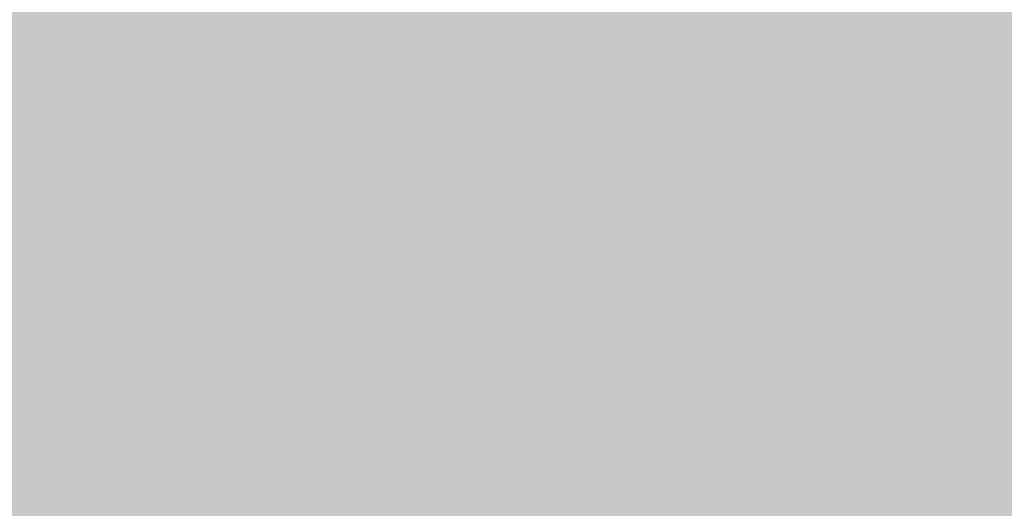
# Model space of a CAD drawing. Units: inches. Extents: x 2083 to 3317, y 1141 to 2115.
# Tile 159 of 256: x 3126.955939 to 3126.958245, y 1263.262504 to 1263.263648. Entities that reach past the tile are written whole.
import ezdxf

# ---------------------------------------------------------------- set-up
doc = ezdxf.new("R2010")
doc.units = ezdxf.units.IN
doc.layers.add('A-WALL-PATT', color=251, linetype='Continuous', lineweight=13, true_color=0x636466)

msp = doc.modelspace()

# ---------------------------------------------------------------- hatches: boundary and pattern name
at = {"layer": 'A-WALL-PATT'}
h = msp.add_hatch(color=256, dxfattribs=at)
h.dxf.hatch_style = 1
h.paths.add_polyline_path([(3126.9597832, 2020.7613601), (2748.9597832, 2020.7613601), (2604.9597832, 2020.7613601), (2226.9597832, 2020.7613601), (2226.9597832, 1702.7613601), (2466.9597832, 1702.7613601), (2466.9597832, 1582.7613601), (2418.9597832, 1582.7613601), (2418.9597832, 1477.7613601), (2226.9597832, 1477.7613601), (2226.9597832, 1263.2613601), (2544.9597832, 1263.2613601), (2544.9597832, 1411.7613601), (2604.9597832, 1411.7613601), (2685.9597832, 1411.7613601), (2685.9597832, 1420.7613601), (2604.9597832, 1420.7613601), (2604.9597832, 1573.7613601), (2604.9597832, 1702.7613601), (2604.9597832, 2011.7613601), (2748.9597832, 2011.7613601), (2748.9597832, 1702.7613601), (2862.9597832, 1702.7613601), (2862.9597832, 1621.7613601), (2871.9597832, 1621.7613601), (2871.9597832, 1702.7613601), (2883.9597832, 1702.7613601), (2883.9597832, 1706.9394595, -0.026459), (2883.9597832, 1711.7613601), (2757.9597832, 1711.7613601), (2757.9597832, 1807.7613601), (2787.9597832, 1807.7613601), (2787.9597832, 1812.2613601), (2757.9597832, 1812.2613601), (2757.9597832, 2011.7613601), (2877.9597832, 2011.7613601), (2877.9597832, 1812.2613601), (2847.9597832, 1812.2613601), (2847.9597832, 1807.7613601), (2889.8357425, 1807.7613601), (2889.8357425, 1812.2613601), (2882.4597832, 1812.2613601), (2882.4597832, 2011.7613601), (3117.9597832, 2011.7613601), (3117.9597832, 1812.2613601), (2937.8357425, 1812.2613601), (2937.8357425, 1807.7613601), (2995.7097832, 1807.7613601), (2995.7097832, 1796.1176655), (3000.2097832, 1796.1176655), (3000.2097832, 1807.7613601), (3117.9597832, 1807.7613601), (3117.9597832, 1711.7613601), (3000.2097832, 1711.7613601), (3000.2097832, 1760.1176655), (2998.5727047, 1760.1176655, -0.020711), (2995.7097832, 1760.1176655), (2995.7097832, 1711.7613601), (2931.9597832, 1711.7613601), (2931.9597832, 1702.7613601), (3126.9597832, 1702.7613601)])
h.paths.add_polyline_path([(2471.4597832, 2011.7613601), (2471.4597832, 1810.0113601), (2462.7169357, 1810.0113601), (2462.7169357, 1805.5113601), (2505.9597832, 1805.5113601), (2505.9597832, 1810.0113601), (2475.9597832, 1810.0113601), (2475.9597832, 2011.7613601), (2595.9597832, 2011.7613601), (2595.9597832, 1810.0113601), (2565.9597832, 1810.0113601), (2565.9597832, 1805.5113601), (2595.9597832, 1805.5113601), (2595.9597832, 1711.7613601), (2235.9597832, 1711.7613601), (2235.9597832, 1805.5113601), (2353.7097832, 1805.5113601), (2353.7097832, 1796.0541624), (2358.2097832, 1796.0541624), (2358.2097832, 1805.5113601), (2414.7169357, 1805.5113601), (2414.7169357, 1810.0113601), (2235.9597832, 1810.0113601), (2235.9597832, 2011.7613601)], flags=16)
h.paths.add_polyline_path([(2270.2047343, 1994.6100082), (2270.2047343, 1970.6100082), (2246.2047343, 1970.6100082), (2246.2047343, 1994.6100082)], flags=0)
edge = h.paths.add_edge_path(flags=0)
edge.add_ellipse((2332.027391, 1899.7981761), major_axis=(-3.0429938, 3.0429938), ratio=0.16825245, start_angle=-161.3321656, end_angle=-156.3071136, ccw=False)
edge.add_ellipse((2333.0820373, 1898.7435297), major_axis=(-1.0546463, 1.0546463), ratio=0.453532097, start_angle=-123.371019, end_angle=-94.1591066)
edge = h.paths.add_edge_path(flags=0)
edge.add_ellipse((2332.027391, 1968.8762897), major_axis=(3.0429938, 3.0429938), ratio=0.16825245, start_angle=18.6678344, end_angle=23.6928864)
edge.add_spline(control_points=[(2332.9255964, 1970.6911045), (2332.2267681, 1970.3360997), (2330.8937087, 1969.6589054), (2328.4130803, 1970.9321376), (2327.2039345, 1967.7487119), (2324.7095965, 1969.9555886), (2322.5328223, 1967.012354), (2320.0128462, 1971.2958124), (2317.6803077, 1968.1578449), (2316.0405263, 1967.1020468), (2315.4269045, 1966.8096022)], knot_values=[0, 0, 0, 0, 2.267059, 4.324559, 6.685584, 8.878641, 11.121502, 14.300359, 17.755284, 19.732645, 19.732645, 19.732645, 19.732645], degree=3, periodic=0)
edge.add_ellipse((2332.027391, 1968.8762897), major_axis=(3.0429938, 3.0429938), ratio=0.16825245, start_angle=18.6678344, end_angle=23.6928864, ccw=False)
edge.add_ellipse((2333.0820373, 1969.930936), major_axis=(1.0546463, 1.0546463), ratio=0.453532097, start_angle=56.628981, end_angle=85.8408934, ccw=False)
edge = h.paths.add_edge_path(flags=0)
edge.add_spline(control_points=[(2296.4282874, 1967.9879081), (2293.6278045, 1965.3363137), (2287.7036238, 1959.727094), (2299.7438601, 1949.9956993), (2294.5325909, 1935.6685275), (2290.5732281, 1920.6035119), (2293.3941244, 1909.9736911), (2296.1854073, 1904.9665431)], knot_values=[0.099185, 0.099185, 0.099185, 0.099185, 0.345301, 0.619822, 0.982653, 1.386093, 1.810555, 1.810555, 1.810555, 1.810555], degree=3, periodic=0)
edge.add_spline(control_points=[(2296.1854073, 1904.9665431), (2297.3835817, 1902.6193002), (2298.0009694, 1901.9493116), (2298.5529698, 1901.4681549)], knot_values=[0.006246, 0.006246, 0.006246, 0.006246, 0.055476, 0.055476, 0.055476, 0.055476], degree=3, periodic=0)
edge.add_spline(control_points=[(2298.5529698, 1901.4681549), (2297.2586121, 1900.9232238), (2295.2252939, 1900.2321257), (2293.0602287, 1900.6142053), (2292.1014227, 1900.788415), (2292.0895776, 1900.790568)], knot_values=[0.312835, 0.312835, 0.312835, 0.312835, 0.40178, 0.474987, 0.475903, 0.475903, 0.475903, 0.475903], degree=3, periodic=0)
edge.add_arc((2292.7936464, 1904.6641088), 3.9370079, 215.4208969, 259.6981795, ccw=False)
edge.add_spline(control_points=[(2289.5853139, 1902.3823039), (2289.4766524, 1902.5350874), (2289.3684805, 1902.6880353), (2289.2608648, 1902.8411699)], knot_values=[0.102872, 0.102872, 0.102872, 0.102872, 0.116896, 0.116896, 0.116896, 0.116896], degree=3, periodic=0)
edge.add_spline(control_points=[(2289.2608648, 1902.8411699), (2288.6866042, 1902.5501922), (2287.6400477, 1902.0199025), (2285.8813368, 1901.8739536), (2283.8529717, 1901.5043521), (2281.7199871, 1899.7105375), (2278.4669913, 1899.492942), (2276.1571361, 1901.8832022), (2272.2589526, 1899.8040711), (2267.7776054, 1901.8431828), (2262.2438819, 1900.1840326), (2257.414927, 1901.7820606), (2254.318374, 1900.7261196), (2253.1782849, 1900.3373431)], knot_values=[0, 0, 0, 0, 1.907977, 3.477176, 5.261074, 7.972851, 11.680248, 13.717921, 16.939592, 22.789562, 27.502503, 33.595215, 37.145618, 37.145618, 37.145618, 37.145618], degree=3, periodic=0)
edge.add_line((2253.1782849, 1900.3373431), (2250.2442397, 1902.8411699))
edge.add_line((2250.2442397, 1902.8411699), (2250.2442397, 1965.8332959))
edge.add_line((2250.2442397, 1965.8332959), (2253.1782849, 1968.3371226))
edge.add_spline(control_points=[(2253.1782849, 1968.3371226), (2254.318374, 1967.9483462), (2257.414927, 1966.8924051), (2262.2438819, 1968.4904332), (2267.7776054, 1966.8312829), (2271.5267301, 1968.5372172), (2273.8759143, 1967.8282895), (2274.2067012, 1967.7276424)], knot_values=[0, 0, 0, 0, 0.09018, 0.244935, 0.364644, 0.513233, 0.537855, 0.537855, 0.537855, 0.537855], degree=3, periodic=0)
edge.add_arc((2274.3528869, 1963.7933495), 3.9370079, 72.0511336, 92.1279492, ccw=False)
edge.add_arc((2281.2969331, 1985.2300027), 18.5962982, 252.05113361, 288.56572166)
edge.add_arc((2292.3167172, 1956.0288805), 12.6460805, 71.02678788, 113.77821843, ccw=False)
edge = h.paths.add_edge_path(flags=0)
edge.add_spline(control_points=[(2274.8994147, 1951.8561946), (2275.066156, 1951.6165924), (2275.2326866, 1951.3765878), (2275.3979871, 1951.1358545)], knot_values=[1.409916, 1.409916, 1.409916, 1.409916, 1.43159, 1.43159, 1.43159, 1.43159], degree=3, periodic=0)
edge.add_spline(control_points=[(2275.3979871, 1951.1358545), (2275.7921055, 1950.5618854), (2276.1792311, 1949.9837745), (2276.5455462, 1949.3971029)], knot_values=[1.358238, 1.358238, 1.358238, 1.358238, 1.409916, 1.409916, 1.409916, 1.409916], degree=3, periodic=0)
edge.add_line((2276.5455462, 1949.3971029), (2277.437289, 1947.8621847))
edge.add_spline(control_points=[(2277.437289, 1947.8621847), (2276.3038341, 1945.6731147), (2274.6396979, 1942.4268817), (2274.631615, 1938.0938998), (2272.7991237, 1930.8515498), (2274.3564261, 1943.8970461), (2275.9476814, 1947.9233558), (2276.5455462, 1949.3971029)], knot_values=[0.005632, 0.005632, 0.005632, 0.005632, 0.186014, 0.266002, 0.357087, 0.59639, 0.739732, 0.739732, 0.739732, 0.739732], degree=3, periodic=0)
edge.add_spline(control_points=[(2276.5455462, 1949.3971029), (2276.1792311, 1949.9837745), (2275.7921055, 1950.5618854), (2275.3979871, 1951.1358545)], knot_values=[1.358238, 1.358238, 1.358238, 1.358238, 1.409916, 1.409916, 1.409916, 1.409916], degree=3, periodic=0)
edge.add_spline(control_points=[(2275.3979871, 1951.1358545), (2274.9425002, 1950.0804523), (2274.2077604, 1948.0252718), (2273.9346018, 1944.8514774), (2272.4685341, 1937.6274891), (2273.4662155, 1945.6964663), (2274.7006154, 1951.0594725), (2274.8994147, 1951.8561946)], knot_values=[0.104364, 0.104364, 0.104364, 0.104364, 0.189636, 0.269624, 0.36071, 0.600013, 0.644622, 0.644622, 0.644622, 0.644622], degree=3, periodic=0)
h.paths.add_polyline_path([(2269.1675139, 1963.1275729, -0.357527), (2268.170633, 1960.9763695, -0.092561), (2268.170633, 1939.4363249, -0.357527), (2269.1675139, 1937.2851215, -0.357527), (2267.0163105, 1938.2820024, -0.164785), (2254.6855813, 1938.2820024, -0.357527), (2252.5343779, 1937.2851215, -0.357527), (2253.5312587, 1939.4363249, -0.092561), (2253.5312587, 1960.9763695, -0.357527), (2252.5343779, 1963.1275729, -0.357527), (2254.6855813, 1962.130692, -0.164785), (2267.0163105, 1962.130692, -0.357527)], flags=0)
h.paths.add_polyline_path([(2248.8740679, 1967.8017998), (2248.8740679, 1957.0277095), (2249.4577833, 1957.0277095), (2249.4577833, 1911.6467562), (2248.8740679, 1911.6467562), (2248.8740679, 1900.8726659), (2246.5118632, 1900.8726659, 0.197327), (2244.1496584, 1902.4568734), (2244.1496584, 1966.2175923, 0.197327), (2246.5118632, 1967.8017998)], flags=0)
h.paths.add_polyline_path([(2269.1675139, 1931.3893442, -0.357527), (2268.170633, 1929.2381408, -0.092561), (2268.170633, 1907.6980962, -0.357527), (2269.1675139, 1905.5468928, -0.357527), (2267.0163105, 1906.5437737, -0.164785), (2254.6855813, 1906.5437737, -0.357527), (2252.5343779, 1905.5468928, -0.357527), (2253.5312587, 1907.6980962, -0.092561), (2253.5312587, 1929.2381408, -0.357527), (2252.5343779, 1931.3893442, -0.357527), (2254.6855813, 1930.3924634, -0.164785), (2267.0163105, 1930.3924634, -0.357527)], flags=0)
edge = h.paths.add_edge_path(flags=0)
edge.add_spline(control_points=[(2276.1968578, 1906.7237016), (2276.1681442, 1909.0289278), (2276.1140492, 1913.371852), (2270.5984171, 1924.9249783), (2273.9051746, 1919.0127787), (2275.9217115, 1916.2620626), (2275.4745699, 1912.4021495), (2277.2578735, 1910.3806206), (2276.6960436, 1908.2250358), (2276.6462176, 1906.8130226), (2276.6178249, 1906.0084068)], knot_values=[0, 0, 0, 0, 8.61026, 16.221274, 18.843057, 23.804898, 27.440828, 29.356102, 31.203478, 33.650687, 33.650687, 33.650687, 33.650687], degree=3, periodic=0)
edge.add_spline(control_points=[(2276.6178249, 1906.0084068), (2276.6233131, 1905.6241436), (2276.4977381, 1904.6286608), (2275.4417789, 1903.8547251), (2274.9373144, 1903.0804497), (2274.8590804, 1902.8411699)], knot_values=[0.156488, 0.156488, 0.156488, 0.156488, 0.184398, 0.231376, 0.250598, 0.250598, 0.250598, 0.250598], degree=3, periodic=0)
edge.add_line((2274.8590804, 1902.8411699), (2276.50598, 1902.8411699))
edge.add_spline(control_points=[(2276.50598, 1902.8411699), (2276.7883084, 1903.0849395), (2277.6650711, 1904.1251958), (2278.2495378, 1904.340738), (2277.6538719, 1908.5273866), (2278.15567, 1906.2278078), (2278.100464, 1905.2859484), (2278.8466748, 1904.0690054), (2277.8567853, 1903.4149482), (2277.8741909, 1902.9910497), (2277.9035616, 1902.8411699)], knot_values=[0.059574, 0.059574, 0.059574, 0.059574, 0.080753, 0.103741, 0.16972, 0.176036, 0.207137, 0.240474, 0.262341, 0.27366, 0.27366, 0.27366, 0.27366], degree=3, periodic=0)
edge.add_line((2277.9035616, 1902.8411699), (2280.0298255, 1902.8411699))
edge.add_spline(control_points=[(2280.0298255, 1902.8411699), (2279.8882214, 1903.088398), (2279.4992571, 1903.9815512), (2280.1522839, 1905.9393491), (2278.103615, 1909.6577572), (2279.7623946, 1907.185285), (2280.3279002, 1904.8748608), (2280.4851086, 1903.4895904), (2281.4632687, 1903.2494323), (2281.7583431, 1902.9364967), (2281.8340361, 1902.8411699)], knot_values=[0.013856, 0.013856, 0.013856, 0.013856, 0.034874, 0.088867, 0.107879, 0.126738, 0.158714, 0.193757, 0.217487, 0.226722, 0.226722, 0.226722, 0.226722], degree=3, periodic=0)
edge.add_spline(control_points=[(2281.8340361, 1902.8411699), (2281.7875348, 1902.8267029), (2281.6470224, 1902.7829881), (2281.3955272, 1902.85949), (2281.088077, 1902.9852418), (2280.7206826, 1903.060902), (2280.3334513, 1903.0257257), (2280.1247668, 1902.898879), (2280.0298255, 1902.8411699)], knot_values=[0, 0, 0, 0, 0.14413, 0.435517, 0.749276, 1.153046, 1.548371, 1.878348, 1.878348, 1.878348, 1.878348], degree=3, periodic=0)
edge.add_line((2280.0298255, 1902.8411699), (2277.9035616, 1902.8411699))
edge.add_spline(control_points=[(2277.9035616, 1902.8411699), (2277.892855, 1902.7958553), (2277.865396, 1902.6796374), (2277.6074793, 1902.6874828), (2277.2740503, 1902.8006999), (2276.8379209, 1902.6197745), (2276.5838074, 1902.7892611), (2276.50598, 1902.8411699)], knot_values=[0, 0, 0, 0, 0.127189, 0.326199, 0.628009, 1.24357, 1.515331, 1.515331, 1.515331, 1.515331], degree=3, periodic=0)
edge.add_line((2276.50598, 1902.8411699), (2274.8590804, 1902.8411699))
edge.add_spline(control_points=[(2274.8590804, 1902.8411699), (2274.8144367, 1902.8985868), (2274.7251297, 1903.013446), (2274.4934765, 1903.1189684), (2274.2442854, 1902.9605386), (2273.9371207, 1903.1849416), (2273.6140395, 1902.9831428), (2273.4083164, 1902.8830449), (2273.322254, 1902.8411699)], knot_values=[0, 0, 0, 0, 0.21843, 0.436957, 0.687977, 0.990379, 1.398396, 1.69185, 1.69185, 1.69185, 1.69185], degree=3, periodic=0)
edge.add_spline(control_points=[(2273.322254, 1902.8411699), (2273.6167403, 1903.445692), (2274.2739977, 1904.5382529), (2276.0272387, 1904.5737017), (2276.2069634, 1906.5836372), (2276.1968578, 1906.7237016)], knot_values=[0.012227, 0.012227, 0.012227, 0.012227, 0.059472, 0.106218, 0.134458, 0.134458, 0.134458, 0.134458], degree=3, periodic=0)
h.paths.add_polyline_path([(2270.7760538, 1897.7898284), (2270.7760538, 1873.7898284), (2246.7760538, 1873.7898284), (2246.7760538, 1897.7898284)], flags=0)
h.paths.add_polyline_path([(2353.7097832, 1760.0050593), (2353.7097832, 1760.0541624), (2358.2097832, 1760.0541624, -0.033729)], flags=0)
h.paths.add_polyline_path([(2321.8191188, 1737.5291862), (2341.9953271, 1737.5291862, -0.414214), (2343.2032727, 1736.3212406), (2343.2032727, 1721.0205964, -0.414214), (2341.9953271, 1719.8126508), (2321.8191188, 1719.8126508, -0.414214), (2320.6111732, 1721.0205964), (2320.6111732, 1736.3212406, -0.414214)], flags=0)
h.paths.add_polyline_path([(2324.2350099, 1736.3212406), (2339.5794359, 1736.3212406, -0.414214), (2341.9953271, 1733.9053494), (2341.9953271, 1725.4497302, -0.414214), (2339.5794359, 1723.033839), (2333.6805885, 1723.033839), (2333.8453172, 1722.0454666, -0.870646), (2335.4253988, 1721.8258934, -0.767327), (2333.922694, 1721.4232449), (2331.2910241, 1721.4232449, -0.767327), (2329.7883193, 1721.8258934, -0.870646), (2331.3684009, 1722.0454666), (2331.5331296, 1723.033839), (2324.2350099, 1723.033839, -0.414214), (2321.8191188, 1725.4497302), (2321.8191188, 1733.9053494, -0.414214)], flags=0)
h.paths.add_polyline_path([(2570.4837892, 1928.6154443), (2589.6837892, 1928.6154443), (2590.1688286, 1928.6154443), (2590.1688286, 1904.9933971), (2570.4837892, 1904.9933971)], flags=0)
h.paths.add_polyline_path([(2574.4473242, 1927.2638215, -1), (2572.8288357, 1927.2638215, -1)], flags=0)
h.paths.add_polyline_path([(2573.0898665, 1926.9408768), (2573.925032, 1927.7760423), (2574.1477428, 1927.5533315), (2573.3125773, 1926.718166)], flags=0)
h.paths.add_polyline_path([(2578.7790648, 1919.7296175, -1), (2571.5916632, 1919.7296175, -1)], flags=0)
h.paths.add_polyline_path([(2578.385364, 1919.7296175, -1), (2571.985364, 1919.7296175, -1)], flags=0)
h.paths.add_polyline_path([(2331.5957638, 1729.4762156, -1), (2333.6179542, 1729.4762156, -1)], flags=0)
h.paths.add_polyline_path([(2578.0342282, 1927.2638215, -1), (2576.4157396, 1927.2638215, -1)], flags=0)
h.paths.add_polyline_path([(2576.6888513, 1927.5310886), (2576.9115621, 1927.7537993), (2577.7467276, 1926.9186339), (2577.5240168, 1926.6959231)], flags=0)
h.paths.add_polyline_path([(2578.1390648, 1909.8595388, -1), (2572.2316632, 1909.8595388, -1)], flags=0)
h.paths.add_polyline_path([(2577.745364, 1909.8595388, -1), (2572.625364, 1909.8595388, -1)], flags=0)
h.paths.add_polyline_path([(2583.7977179, 1927.2638215, -1), (2582.1792294, 1927.2638215, -1)], flags=0)
h.paths.add_polyline_path([(2582.7186487, 1927.7537993), (2583.5538142, 1926.9186339), (2583.3311034, 1926.6959231), (2582.4959379, 1927.5310886)], flags=0)
h.paths.add_polyline_path([(2582.4959379, 1927.5310886), (2582.7186487, 1927.7537993), (2583.5538142, 1926.9186339), (2583.3311034, 1926.6959231)], flags=0)
h.paths.add_polyline_path([(2587.7390648, 1920.5296175, -1), (2581.8316632, 1920.5296175, -1)], flags=0)
h.paths.add_polyline_path([(2587.345364, 1920.5296175, -1), (2582.225364, 1920.5296175, -1)], flags=0)
h.paths.add_polyline_path([(2587.3846219, 1927.2638215, -1), (2585.7661333, 1927.2638215, -1)], flags=0)
h.paths.add_polyline_path([(2586.0819925, 1926.9802469), (2586.917158, 1927.8154124), (2587.1398688, 1927.5927016), (2586.3047033, 1926.7575361)], flags=0)
h.paths.add_polyline_path([(2588.3790648, 1910.6595388, -1), (2581.1916632, 1910.6595388, -1)], flags=0)
h.paths.add_polyline_path([(2587.985364, 1910.6595388, -1), (2581.585364, 1910.6595388, -1)], flags=0)
h.paths.add_polyline_path([(2417.1677288, 1729.4778955), (2437.3439372, 1729.4778955, -0.414214), (2438.5518828, 1728.2699499), (2438.5518828, 1712.9693057, -0.414214), (2437.3439372, 1711.7613601), (2417.1677288, 1711.7613601, -0.414214), (2415.9597832, 1712.9693057), (2415.9597832, 1728.2699499, -0.414214)], flags=0)
h.paths.add_polyline_path([(2419.58362, 1728.2699499), (2434.928046, 1728.2699499, -0.414214), (2437.3439372, 1725.8540587), (2437.3439372, 1717.3984395, -0.414214), (2434.928046, 1714.9825483), (2429.0291985, 1714.9825483), (2429.1939273, 1713.9941758, -0.870646), (2430.7740089, 1713.7746027, -0.767327), (2429.2713041, 1713.3719542), (2426.6396342, 1713.3719542, -0.767327), (2425.1369294, 1713.7746027, -0.870646), (2426.717011, 1713.9941758), (2426.8817397, 1714.9825483), (2419.58362, 1714.9825483, -0.414214), (2417.1677288, 1717.3984395), (2417.1677288, 1725.8540587, -0.414214)], flags=0)
h.paths.add_polyline_path([(2419.58362, 1728.2699499), (2434.928046, 1728.2699499, -0.414214), (2437.3439372, 1725.8540587), (2437.3439372, 1717.3984395, -0.414214), (2434.928046, 1714.9825483), (2429.0291985, 1714.9825483), (2428.3581177, 1719.0090337), (2427.5528206, 1719.0090337), (2426.8817397, 1714.9825483), (2419.58362, 1714.9825483, -0.414214), (2417.1677288, 1717.3984395), (2417.1677288, 1725.8540587, -0.414214)], flags=0)
h.paths.add_polyline_path([(2426.9443739, 1721.4249248, -1), (2428.9665643, 1721.4249248, -1)], flags=0)
h.paths.add_polyline_path([(2475.9597832, 1702.7613601), (2595.9597832, 1702.7613601), (2595.9597832, 1582.7613601), (2475.9597832, 1582.7613601)], flags=16)
h.paths.add_polyline_path([(2427.9597832, 1573.7613601), (2595.9597832, 1573.7613601), (2595.9597832, 1468.7613601), (2595.9597832, 1420.7613601), (2384.4597832, 1420.7613601), (2384.4597832, 1468.7613601), (2427.9597832, 1468.7613601)], flags=16)
h.paths.add_polyline_path([(2379.9597832, 1468.7613601), (2379.9597832, 1420.7613601), (2235.9597832, 1420.7613601), (2235.9597832, 1468.7613601)], flags=16)
h.paths.add_polyline_path([(2317.8159962, 1466.695767), (2337.9922045, 1466.695767, -0.414214), (2339.2001501, 1465.4878214), (2339.2001501, 1450.1871771, -0.414214), (2337.9922045, 1448.9792315), (2317.8159962, 1448.9792315, -0.414214), (2316.6080506, 1450.1871771), (2316.6080506, 1465.4878214, -0.414214)], flags=0)
h.paths.add_polyline_path([(2320.2318874, 1465.4878214), (2335.5763133, 1465.4878214, -0.414214), (2337.9922045, 1463.0719302), (2337.9922045, 1454.616311, -0.414214), (2335.5763133, 1452.2004198), (2329.6774659, 1452.2004198), (2329.8421946, 1451.2120473, -0.870646), (2331.4222762, 1450.9924742, -0.767327), (2329.9195714, 1450.5898257), (2327.2879015, 1450.5898257, -0.767327), (2325.7851967, 1450.9924742, -0.870646), (2327.3652783, 1451.2120473), (2327.530007, 1452.2004198), (2320.2318874, 1452.2004198, -0.414214), (2317.8159962, 1454.616311), (2317.8159962, 1463.0719302, -0.414214)], flags=0)
h.paths.add_polyline_path([(2320.2318874, 1465.4878214), (2335.5763133, 1465.4878214, -0.414214), (2337.9922045, 1463.0719302), (2337.9922045, 1454.616311, -0.414214), (2335.5763133, 1452.2004198), (2329.6774659, 1452.2004198), (2329.006385, 1456.2269051), (2328.2010879, 1456.2269051), (2327.530007, 1452.2004198), (2320.2318874, 1452.2004198, -0.414214), (2317.8159962, 1454.616311), (2317.8159962, 1463.0719302, -0.414214)], flags=0)
h.paths.add_polyline_path([(2327.5926413, 1458.6427963, -1), (2329.6148317, 1458.6427963, -1)], flags=0)
h.paths.add_polyline_path([(2244.4117436, 1433.3404531), (2241.9209449, 1433.3404531, -0.414214), (2240.0178562, 1435.2435418), (2240.0178562, 1440.9528078, -0.414211), (2241.920925, 1442.8558965), (2244.4117436, 1442.8558965, -1.976472)], flags=0)
h.paths.add_polyline_path([(2245.3568884, 1434.3975358, -0.414214), (2245.3568884, 1441.7988138, -2.144098)], flags=0)
h.paths.add_polyline_path([(2535.9597832, 1416.2613601), (2535.9597832, 1272.2613601), (2235.9597832, 1272.2613601), (2235.9597832, 1416.2613601)], flags=16)
h.paths.add_polyline_path([(2260.1195614, 1384.2928413), (2260.1195614, 1362.0386487), (2237.8653688, 1362.0386487), (2237.8653688, 1384.2928413)], flags=0)
edge = h.paths.add_edge_path(flags=0)
edge.add_line((2318.2518466, 1362.0932983), (2318.1457968, 1362.0009726))
edge.add_ellipse((2317.4451158, 1360.4310442), major_axis=(2.8216404, 2.8216404), ratio=0.16825245, start_angle=18.6678344, end_angle=20.9481273, ccw=False)
edge.add_ellipse((2318.4230451, 1361.4089735), major_axis=(0.9779293, 0.9779293), ratio=0.453532097, start_angle=56.628981, end_angle=70.2262012, ccw=False)
edge = h.paths.add_edge_path(flags=0)
edge.add_line((2319.1073699, 1295.5710784), (2319.0150442, 1295.6771282))
edge.add_ellipse((2317.4451158, 1296.3778091), major_axis=(-2.8216404, 2.8216404), ratio=0.16825245, start_angle=-161.3321656, end_angle=-159.0518727, ccw=False)
edge.add_ellipse((2318.4230451, 1295.3998798), major_axis=(-0.9779293, 0.9779293), ratio=0.453532097, start_angle=-123.371019, end_angle=-109.7737988)
edge = h.paths.add_edge_path(flags=0)
edge.add_spline(control_points=[(2284.2103489, 1301.1702189), (2284.5806878, 1300.444719), (2284.8911891, 1299.8920243), (2285.159553, 1299.4610182)], knot_values=[0.039066, 0.039066, 0.039066, 0.039066, 0.055476, 0.055476, 0.055476, 0.055476], degree=3, periodic=0)
edge.add_line((2285.159553, 1299.4610182), (2284.2103489, 1301.1702189))
edge = h.paths.add_edge_path(flags=0)
edge.add_line((2280.4124579, 1297.2980125), (2283.3699905, 1297.0361216))
edge.add_line((2283.3699905, 1297.0361216), (2286.4056902, 1297.9263104))
edge.add_spline(control_points=[(2286.4056902, 1297.9263104), (2285.305487, 1297.4631193), (2284.3447774, 1297.1291508), (2283.3699905, 1297.0361216)], knot_values=[0.394369, 0.394369, 0.394369, 0.394369, 0.475903, 0.475903, 0.475903, 0.475903], degree=3, periodic=0)
edge.add_spline(control_points=[(2283.3699905, 1297.0361216), (2283.2813895, 1297.027666), (2282.316289, 1296.9573356), (2281.3125019, 1297.1344787), (2280.4234414, 1297.2960161), (2280.4124579, 1297.2980125)], knot_values=[0.312835, 0.312835, 0.312835, 0.312835, 0.320246, 0.393453, 0.394369, 0.394369, 0.394369, 0.394369], degree=3, periodic=0)
edge = h.paths.add_edge_path(flags=0)
edge.add_line((2284.4355615, 1359.6072854), (2280.4462909, 1355.328047))
edge.add_line((2280.4462909, 1355.328047), (2279.5799868, 1351.0177544))
edge.add_line((2279.5799868, 1351.0177544), (2282.4129737, 1346.5804327))
edge.add_spline(control_points=[(2282.4129737, 1346.5804327), (2283.1533308, 1345.5892358), (2284.2528957, 1344.0288973), (2284.801037, 1342.3871671), (2284.9351625, 1341.8055443)], knot_values=[1.240098, 1.240098, 1.240098, 1.240098, 1.332892, 1.382712, 1.382712, 1.382712, 1.382712], degree=3, periodic=0)
edge.add_spline(control_points=[(2284.9351625, 1341.8055443), (2285.3191079, 1340.1406002), (2285.2330291, 1338.4092041), (2284.9099384, 1336.6541222)], knot_values=[1.097484, 1.097484, 1.097484, 1.097484, 1.240098, 1.240098, 1.240098, 1.240098], degree=3, periodic=0)
edge.add_spline(control_points=[(2284.9099384, 1336.6541222), (2284.5868478, 1334.8990403), (2284.0267453, 1333.1202725), (2283.4626437, 1331.3605849)], knot_values=[0.95487, 0.95487, 0.95487, 0.95487, 1.097484, 1.097484, 1.097484, 1.097484], degree=3, periodic=0)
edge.add_line((2283.4626437, 1331.3605849), (2281.8903759, 1326.153357))
edge.add_line((2281.8903759, 1326.153357), (2280.7562592, 1321.0560888))
edge.add_line((2280.7562592, 1321.0560888), (2280.2992048, 1316.0019772))
edge.add_line((2280.2992048, 1316.0019772), (2280.7159327, 1310.9500678))
edge.add_line((2280.7159327, 1310.9500678), (2282.0280939, 1305.9721367))
edge.add_line((2282.0280939, 1305.9721367), (2284.2103489, 1301.1702189))
edge.add_spline(control_points=[(2284.2103489, 1301.1702189), (2283.3407305, 1302.7301854), (2282.6119044, 1304.3364933), (2282.0280939, 1305.9721367)], knot_values=[0.099185, 0.099185, 0.099185, 0.099185, 0.241799, 0.241799, 0.241799, 0.241799], degree=3, periodic=0)
edge.add_spline(control_points=[(2282.0280939, 1305.9721367), (2281.4442835, 1307.6077801), (2281.0054886, 1309.2727591), (2280.7159327, 1310.9500678)], knot_values=[0.241799, 0.241799, 0.241799, 0.241799, 0.384413, 0.384413, 0.384413, 0.384413], degree=3, periodic=0)
edge.add_spline(control_points=[(2280.7159327, 1310.9500678), (2280.4332411, 1312.5876134), (2280.2893863, 1314.2769594), (2280.2988938, 1315.9620324), (2280.2992048, 1316.0019772)], knot_values=[0.384413, 0.384413, 0.384413, 0.384413, 0.523647, 0.527028, 0.527028, 0.527028, 0.527028], degree=3, periodic=0)
edge.add_spline(control_points=[(2280.2992048, 1316.0019772), (2280.3123257, 1317.6869552), (2280.4778706, 1319.3679256), (2280.7562592, 1321.0560888)], knot_values=[0.527028, 0.527028, 0.527028, 0.527028, 0.669642, 0.669642, 0.669642, 0.669642], degree=3, periodic=0)
edge.add_spline(control_points=[(2280.7562592, 1321.0560888), (2281.0346478, 1322.7442519), (2281.4258801, 1324.4396079), (2281.8903759, 1326.153357)], knot_values=[0.669642, 0.669642, 0.669642, 0.669642, 0.812256, 0.812256, 0.812256, 0.812256], degree=3, periodic=0)
edge.add_spline(control_points=[(2281.8903759, 1326.153357), (2282.2643834, 1327.5332507), (2282.7878702, 1329.2618097), (2283.352751, 1331.0177803), (2283.4626437, 1331.3605849)], knot_values=[0.812256, 0.812256, 0.812256, 0.812256, 0.927087, 0.95487, 0.95487, 0.95487, 0.95487], degree=3, periodic=0)
edge.add_line((2283.4626437, 1331.3605849), (2284.9099384, 1336.6541222))
edge.add_line((2284.9099384, 1336.6541222), (2284.9351625, 1341.8055443))
edge.add_line((2284.9351625, 1341.8055443), (2282.4129737, 1346.5804327))
edge.add_spline(control_points=[(2282.4129737, 1346.5804327), (2281.2751273, 1348.1037918), (2280.0784467, 1349.5703178), (2279.5799868, 1351.0177544)], knot_values=[1.382712, 1.382712, 1.382712, 1.382712, 1.525326, 1.525326, 1.525326, 1.525326], degree=3, periodic=0)
edge.add_spline(control_points=[(2279.5799868, 1351.0177544), (2279.4432818, 1351.4147209), (2279.1363124, 1352.856922), (2279.7351897, 1354.2903851), (2280.4462909, 1355.328047)], knot_values=[1.525326, 1.525326, 1.525326, 1.525326, 1.564439, 1.667941, 1.667941, 1.667941, 1.667941], degree=3, periodic=0)
edge.add_spline(control_points=[(2280.4462909, 1355.328047), (2281.4261132, 1356.7578354), (2282.9308373, 1358.1825604), (2284.4355615, 1359.6072854)], knot_values=[1.667941, 1.667941, 1.667941, 1.667941, 1.810555, 1.810555, 1.810555, 1.810555], degree=3, periodic=0)
edge.add_arc((2280.6230749, 1348.518181), 11.7261796, 71.02678788, 113.77821843)
edge.add_arc((2270.4048917, 1375.5951559), 17.2435667, 252.05113361, 288.56572166, ccw=False)
edge.add_arc((2263.9659692, 1355.7178471), 3.6506221, 72.0511336, 92.1279492)
edge.add_arc((2263.9659692, 1355.7178471), 3.6506221, 92.1279492, 177.98513)
edge.add_spline(control_points=[(2260.3176041, 1355.8461989), (2260.2604169, 1354.2206683), (2260.551278, 1350.1865469), (2262.9993445, 1346.7662507), (2264.4727415, 1344.6490245)], knot_values=[1.43159, 1.43159, 1.43159, 1.43159, 1.564144, 1.770695, 1.770695, 1.770695, 1.770695], degree=3, periodic=0)
edge.add_line((2264.4727415, 1344.6490245), (2264.9355904, 1343.9825301))
edge.add_spline(control_points=[(2263.8010444, 1340.2481052), (2263.8432379, 1340.5140884), (2264.0672444, 1341.7564652), (2264.5126928, 1343.0024532), (2264.9350468, 1343.9810834)], knot_values=[0.53657, 0.53657, 0.53657, 0.53657, 0.559349, 0.644622, 0.644622, 0.644622, 0.644622], degree=3, periodic=0)
edge.add_spline(control_points=[(2264.9350468, 1343.9810834), (2265.1177715, 1343.7149747), (2265.2988751, 1343.4479058), (2265.4767562, 1343.1793646)], knot_values=[1.384077, 1.384077, 1.384077, 1.384077, 1.409916, 1.409916, 1.409916, 1.409916], degree=3, periodic=0)
edge.add_spline(control_points=[(2265.4767562, 1343.1793646), (2265.6546373, 1342.9108234), (2265.8292958, 1342.64081), (2265.9991301, 1342.368812)], knot_values=[1.358238, 1.358238, 1.358238, 1.358238, 1.384077, 1.384077, 1.384077, 1.384077], degree=3, periodic=0)
edge.add_line((2265.9991301, 1342.368812), (2266.8260057, 1340.9455468))
edge.add_spline(control_points=[(2266.8260057, 1340.9455468), (2268.894401, 1337.0896912), (2271.3981727, 1325.8430009), (2270.5161644, 1310.5685568), (2275.9193759, 1301.860609), (2277.7895113, 1299.1994495)], knot_values=[0.116896, 0.116896, 0.116896, 0.116896, 0.472987, 1.050969, 1.313793, 1.313793, 1.313793, 1.313793], degree=3, periodic=0)
edge.add_spline(control_points=[(2277.7895113, 1299.1994495), (2277.8394051, 1299.1284519), (2277.8894277, 1299.0574975), (2277.9395717, 1298.9865839)], knot_values=[0.109884, 0.109884, 0.109884, 0.109884, 0.116896, 0.116896, 0.116896, 0.116896], degree=3, periodic=0)
edge.add_line((2277.9395717, 1298.9865839), (2277.7888489, 1299.1991139))
edge.add_spline(control_points=[(2277.7888489, 1299.1991139), (2277.2565819, 1298.9294144), (2276.2863504, 1298.4379024), (2275.0393517, 1298.3344186), (2274.3833299, 1298.2388951), (2274.2152543, 1298.209338)], knot_values=[33.12187, 33.12187, 33.12187, 33.12187, 35.029056, 36.598255, 37.144827, 37.144827, 37.144827, 37.144827], degree=3, periodic=0)
edge.add_line((2274.2152543, 1298.209338), (2273.073147, 1297.8929607))
edge.add_spline(control_points=[(2273.073147, 1297.8929607), (2272.3229363, 1297.579784), (2271.0391507, 1296.5105078), (2269.2483948, 1296.2260622), (2268.4231004, 1296.3746543)], knot_values=[26.532584, 26.532584, 26.532584, 26.532584, 29.198919, 31.839101, 31.839101, 31.839101, 31.839101], degree=3, periodic=0)
edge.add_line((2268.4231004, 1296.3746543), (2263.8785014, 1297.4575338))
edge.add_spline(control_points=[(2263.8785014, 1297.4575338), (2263.5560769, 1297.3594345), (2261.8603064, 1296.8386943), (2260.2387805, 1297.2824073), (2258.9334543, 1297.5164611)], knot_values=[15.919551, 15.919551, 15.919551, 15.919551, 16.939592, 21.226067, 21.226067, 21.226067, 21.226067], degree=3, periodic=0)
edge.add_line((2258.9334543, 1297.5164611), (2254.0552332, 1297.3290098))
edge.add_spline(control_points=[(2254.0552332, 1297.3290098), (2253.7555255, 1297.295815), (2252.1136834, 1297.1651738), (2250.4618687, 1297.5442209), (2249.1296862, 1297.6678818)], knot_values=[5.306517, 5.306517, 5.306517, 5.306517, 6.276435, 10.613034, 10.613034, 10.613034, 10.613034], degree=3, periodic=0)
edge.add_line((2249.1296862, 1297.6678818), (2244.3316495, 1296.8777561))
edge.add_line((2244.3316495, 1296.8777561), (2241.6110326, 1299.1994495))
edge.add_line((2241.6110326, 1299.1994495), (2241.6110326, 1357.6094038))
edge.add_line((2241.6110326, 1357.6094038), (2244.3316495, 1359.9310973))
edge.add_line((2244.3316495, 1359.9310973), (2252.7288228, 1359.5426917))
edge.add_spline(control_points=[(2252.7288228, 1359.5426917), (2252.8709387, 1359.5464396), (2253.3057402, 1359.5481716), (2253.7398447, 1359.5142744), (2254.0317419, 1359.4824261)], knot_values=[0.233291, 0.233291, 0.233291, 0.233291, 0.244935, 0.268927, 0.268927, 0.268927, 0.268927], degree=3, periodic=0)
edge.add_line((2254.0317419, 1359.4824261), (2259.5871899, 1359.4163899))
edge.add_spline(control_points=[(2259.5871899, 1359.4163899), (2260.6770676, 1359.6285026), (2262.0731971, 1359.8970025), (2263.5236925, 1359.4592776), (2263.8304173, 1359.3659518)], knot_values=[0.422516, 0.422516, 0.422516, 0.422516, 0.513233, 0.537855, 0.537855, 0.537855, 0.537855], degree=3, periodic=0)
edge.add_arc((2263.9659692, 1355.7178471), 3.6506221, 72.0511336, 92.1279492, ccw=False)
edge.add_arc((2270.4048917, 1375.5951559), 17.2435667, 252.05113361, 288.56572166)
edge.add_arc((2280.6230749, 1348.518181), 11.7261796, 71.02678788, 113.77821843, ccw=False)
h.paths.add_polyline_path([(2240.3405298, 1359.4347149), (2240.3405298, 1349.4443532), (2240.8817846, 1349.4443532), (2240.8817846, 1307.3645001), (2240.3405298, 1307.3645001), (2240.3405298, 1297.3741385), (2238.1501565, 1297.3741385, 0.197327), (2235.9597832, 1298.8431076), (2235.9597832, 1357.9657458, 0.197327), (2238.1501565, 1359.4347149)], flags=0)
h.paths.add_polyline_path([(2259.1577904, 1355.1005005, -0.357527), (2258.2334246, 1353.1057799, -0.092561), (2258.2334246, 1333.1326007, -0.357527), (2259.1577904, 1331.1378801, -0.357527), (2257.1630698, 1332.0622458, -0.164785), (2245.7293022, 1332.0622458, -0.357527), (2243.7345816, 1331.1378801, -0.357527), (2244.6589474, 1333.1326007, -0.092561), (2244.6589474, 1353.1057799, -0.357527), (2243.7345816, 1355.1005005, -0.357527), (2245.7293022, 1354.1761347, -0.164785), (2257.1630698, 1354.1761347, -0.357527)], flags=0)
edge = h.paths.add_edge_path(flags=0)
edge.add_line((2265.9991301, 1342.368812), (2266.8260057, 1340.9455468))
edge.add_line((2266.8260057, 1340.9455468), (2265.3075567, 1337.8140664))
edge.add_line((2265.3075567, 1337.8140664), (2264.358232, 1334.6529388))
edge.add_line((2264.358232, 1334.6529388), (2264.2620123, 1333.7997046))
edge.add_spline(control_points=[(2264.2620123, 1333.7997046), (2264.2083565, 1333.187055), (2264.1620602, 1332.3655252), (2264.0071444, 1331.4139326), (2263.9690487, 1331.2018338)], knot_values=[0.464444, 0.464444, 0.464444, 0.464444, 0.516691, 0.531608, 0.531608, 0.531608, 0.531608], degree=3, periodic=0)
edge.add_spline(control_points=[(2263.9690487, 1331.2018338), (2263.7745349, 1330.1188727), (2263.4243703, 1328.7908386), (2263.2574202, 1328.5306516), (2263.2340282, 1328.5146115)], knot_values=[0.372682, 0.372682, 0.372682, 0.372682, 0.44885, 0.464444, 0.464444, 0.464444, 0.464444], degree=3, periodic=0)
edge.add_spline(control_points=[(2263.2340282, 1328.5146115), (2263.096382, 1328.4202271), (2263.1311696, 1329.3014765), (2263.2749528, 1330.6157493)], knot_values=[0.280919, 0.280919, 0.280919, 0.280919, 0.372682, 0.372682, 0.372682, 0.372682], degree=3, periodic=0)
edge.add_spline(control_points=[(2263.2749528, 1330.6157493), (2263.4187361, 1331.930022), (2263.6715151, 1333.677318), (2263.9698519, 1335.3150268)], knot_values=[0.189157, 0.189157, 0.189157, 0.189157, 0.280919, 0.280919, 0.280919, 0.280919], degree=3, periodic=0)
edge.add_spline(control_points=[(2263.9698519, 1335.3150268), (2264.1004958, 1336.0321917), (2264.4187827, 1337.6219113), (2264.7548476, 1338.8644304), (2264.9474193, 1339.4911244)], knot_values=[0.097394, 0.097394, 0.097394, 0.097394, 0.137578, 0.189157, 0.189157, 0.189157, 0.189157], degree=3, periodic=0)
edge.add_spline(control_points=[(2264.9474193, 1339.4911244), (2265.2900171, 1340.6060546), (2265.6442376, 1341.4939958), (2265.9991301, 1342.368812)], knot_values=[0.005632, 0.005632, 0.005632, 0.005632, 0.097394, 0.097394, 0.097394, 0.097394], degree=3, periodic=0)
h.paths.add_polyline_path([(2259.1577904, 1325.6709733, -0.357527), (2258.2334246, 1323.6762527, -0.092561), (2258.2334246, 1303.7030735, -0.357527), (2259.1577904, 1301.7083529, -0.357527), (2257.1630698, 1302.6327186, -0.164785), (2245.7293022, 1302.6327186, -0.357527), (2243.7345816, 1301.7083529, -0.357527), (2244.6589474, 1303.7030735, -0.092561), (2244.6589474, 1323.6762527, -0.357527), (2243.7345816, 1325.6709733, -0.357527), (2245.7293022, 1324.7466075, -0.164785), (2257.1630698, 1324.7466075, -0.357527)], flags=0)
edge = h.paths.add_edge_path(flags=0)
edge.add_spline(control_points=[(2261.7089377, 1317.3114208), (2261.6794818, 1317.4175798), (2261.7618581, 1317.3885347), (2262.4907358, 1316.0898725), (2262.962185, 1315.3008975)], knot_values=[14.955861, 14.955861, 14.955861, 14.955861, 16.221274, 18.694826, 18.694826, 18.694826, 18.694826], degree=3, periodic=0)
edge.add_spline(control_points=[(2262.962185, 1315.3008975), (2262.9904374, 1315.2536169), (2263.7020958, 1314.0673762), (2264.3489834, 1313.1271533), (2264.7300545, 1312.1641544)], knot_values=[18.694826, 18.694826, 18.694826, 18.694826, 18.843057, 22.433791, 22.433791, 22.433791, 22.433791], degree=3, periodic=0)
edge.add_spline(control_points=[(2264.7300545, 1312.1641544), (2264.8755649, 1311.7964373), (2265.1768733, 1310.7698073), (2265.1430689, 1309.5592623), (2265.2477363, 1308.8241926)], knot_values=[22.433791, 22.433791, 22.433791, 22.433791, 23.804898, 26.172756, 26.172756, 26.172756, 26.172756], degree=3, periodic=0)
edge.add_line((2265.2477363, 1308.8241926), (2265.8507741, 1307.1718879))
edge.add_spline(control_points=[(2265.8507741, 1307.1718879), (2266.0650246, 1306.8216779), (2266.3843872, 1306.3322461), (2266.4244001, 1305.7805489), (2266.4203688, 1305.6112163)], knot_values=[28.062562, 28.062562, 28.062562, 28.062562, 29.356102, 29.911721, 29.911721, 29.911721, 29.911721], degree=3, periodic=0)
edge.add_spline(control_points=[(2266.4203688, 1305.6112163), (2266.4161162, 1305.4325896), (2266.393999, 1305.2499979), (2266.3647773, 1305.0658571)], knot_values=[29.911721, 29.911721, 29.911721, 29.911721, 30.497837, 30.497837, 30.497837, 30.497837], degree=3, periodic=0)
edge.add_line((2266.3647773, 1305.0658571), (2266.0661511, 1302.1362954))
edge.add_spline(control_points=[(2266.0661511, 1302.1362954), (2266.0712401, 1301.7799843), (2265.9980761, 1301.1999847), (2265.6632664, 1300.7589613), (2265.5089084, 1300.5858824)], knot_values=[0.156488, 0.156488, 0.156488, 0.156488, 0.184398, 0.203543, 0.203543, 0.203543, 0.203543], degree=3, periodic=0)
edge.add_line((2265.5089084, 1300.5858824), (2264.4353411, 1299.1994495))
edge.add_line((2264.4353411, 1299.1994495), (2265.962442, 1299.1994495))
edge.add_line((2265.962442, 1299.1994495), (2267.3359898, 1301.1752758))
edge.add_line((2267.3359898, 1301.1752758), (2267.3116668, 1301.9862366))
edge.add_spline(control_points=[(2267.3116668, 1301.9862366), (2267.261111, 1302.8623959), (2267.1602121, 1303.7371316), (2267.2714865, 1303.3258962)], knot_values=[0.126229, 0.126229, 0.126229, 0.126229, 0.166617, 0.166617, 0.166617, 0.166617], degree=3, periodic=0)
edge.add_spline(control_points=[(2267.2714865, 1303.3258962), (2267.2800347, 1303.2943047), (2267.3097851, 1303.1753659), (2267.3734504, 1302.8836084), (2267.4061233, 1302.6828291), (2267.4179259, 1302.6010251)], knot_values=[0.166617, 0.166617, 0.166617, 0.166617, 0.16972, 0.176036, 0.180765, 0.180765, 0.180765, 0.180765], degree=3, periodic=0)
edge.add_spline(control_points=[(2267.7438914, 1300.9875045), (2267.6875832, 1301.1509426), (2267.4805198, 1301.6566644), (2267.4837514, 1302.1447877), (2267.4179259, 1302.6010251)], knot_values=[0.180765, 0.180765, 0.180765, 0.180765, 0.193767, 0.220139, 0.220139, 0.220139, 0.220139], degree=3, periodic=0)
edge.add_line((2267.4179259, 1302.6010251), (2267.7438914, 1300.9875045))
edge.add_spline(control_points=[(2267.7438914, 1300.9875045), (2267.8319608, 1300.7318778), (2267.9320205, 1300.3099042), (2267.5548409, 1299.9745185), (2267.429366, 1299.8292073)], knot_values=[0.220139, 0.220139, 0.220139, 0.220139, 0.240474, 0.25489, 0.25489, 0.25489, 0.25489], degree=3, periodic=0)
edge.add_line((2267.429366, 1299.8292073), (2267.2583608, 1299.1994495))
edge.add_line((2267.2583608, 1299.1994495), (2269.229956, 1299.1994495))
edge.add_spline(control_points=[(2269.229956, 1299.1994495), (2269.0986525, 1299.4286938), (2268.842774, 1300.0162509), (2269.0115749, 1300.9159235), (2268.9467957, 1301.6607397)], knot_values=[0.013856, 0.013856, 0.013856, 0.013856, 0.034874, 0.067073, 0.067073, 0.067073, 0.067073], degree=3, periodic=0)
edge.add_line((2268.9467957, 1301.6607397), (2268.4315815, 1303.6031089))
edge.add_spline(control_points=[(2268.4315815, 1303.6031089), (2268.1755957, 1304.1923747), (2267.5962136, 1305.2512977), (2268.0406981, 1304.6232098), (2268.2513938, 1304.2824205)], knot_values=[0.090155, 0.090155, 0.090155, 0.090155, 0.107879, 0.120289, 0.120289, 0.120289, 0.120289], degree=3, periodic=0)
edge.add_spline(control_points=[(2268.2513938, 1304.2824205), (2268.3608818, 1304.1053294), (2269.0577527, 1302.9179833), (2269.382691, 1301.5904186), (2269.5214051, 1300.7759312), (2269.5752202, 1300.5557836)], knot_values=[0.120289, 0.120289, 0.120289, 0.120289, 0.126738, 0.158714, 0.173506, 0.173506, 0.173506, 0.173506], degree=3, periodic=0)
edge.add_line((2269.5752202, 1300.5557836), (2270.6857984, 1299.4212579))
edge.add_spline(control_points=[(2270.6857984, 1299.4212579), (2270.7672206, 1299.3572512), (2270.8378523, 1299.2814011), (2270.9029248, 1299.1994495)], knot_values=[0.21816, 0.21816, 0.21816, 0.21816, 0.226722, 0.226722, 0.226722, 0.226722], degree=3, periodic=0)
edge.add_line((2270.9372012, 1299.1929131), (2270.9029248, 1299.1994495))
edge.add_spline(control_points=[(2270.9029248, 1299.1994495), (2270.8598061, 1299.1860349), (2270.7295148, 1299.1455), (2270.4963139, 1299.216437), (2270.2716612, 1299.3083234), (2270.1210168, 1299.3479612), (2270.0633386, 1299.3595566)], knot_values=[0.939174, 0.939174, 0.939174, 0.939174, 1.083304, 1.374691, 1.68845, 1.878348, 1.878348, 1.878348, 1.878348], degree=3, periodic=0)
edge.add_line((2270.0633386, 1299.3595566), (2269.229956, 1299.1994495))
edge.add_line((2269.229956, 1299.1994495), (2267.2583608, 1299.1994495))
edge.add_spline(control_points=[(2267.2583608, 1299.1994495), (2267.248433, 1299.1574312), (2267.2229714, 1299.0496673), (2266.9838161, 1299.056942), (2266.8092097, 1299.1162303), (2266.6769047, 1299.1090913), (2266.636531, 1299.1048147)], knot_values=[0.757665, 0.757665, 0.757665, 0.757665, 0.884854, 1.083864, 1.385675, 1.515331, 1.515331, 1.515331, 1.515331], degree=3, periodic=0)
edge.add_spline(control_points=[(2266.636531, 1299.1048147), (2266.4852248, 1299.0887878), (2266.2358066, 1299.0171229), (2266.0346081, 1299.1513168), (2265.962442, 1299.1994495)], knot_values=[0, 0, 0, 0, 0.485905, 0.757665, 0.757665, 0.757665, 0.757665], degree=3, periodic=0)
edge.add_line((2265.962442, 1299.1994495), (2264.4353411, 1299.1994495))
edge.add_line((2264.4353411, 1299.1994495), (2263.8584442, 1299.3671176))
edge.add_spline(control_points=[(2263.8584442, 1299.3671176), (2263.8189433, 1299.3709053), (2263.7795277, 1299.3857212), (2263.7401308, 1299.4015039)], knot_values=[0.845925, 0.845925, 0.845925, 0.845925, 0.978627, 0.978627, 0.978627, 0.978627], degree=3, periodic=0)
edge.add_line((2263.7217862, 1299.3964251), (2263.0103065, 1299.1994495))
edge.add_spline(control_points=[(2263.0103065, 1299.1994495), (2263.2457942, 1299.682859), (2263.5060317, 1300.1281072), (2263.8734943, 1300.4080279)], knot_values=[0.012227, 0.012227, 0.012227, 0.012227, 0.052971, 0.052971, 0.052971, 0.052971], degree=3, periodic=0)
edge.add_spline(control_points=[(2263.8734943, 1300.4080279), (2263.932131, 1300.4526954), (2264.0842429, 1300.5529789), (2264.2551889, 1300.6242227), (2264.3596855, 1300.6647475)], knot_values=[0.052971, 0.052971, 0.052971, 0.052971, 0.059472, 0.069086, 0.069086, 0.069086, 0.069086], degree=3, periodic=0)
edge.add_line((2264.3596855, 1300.6647475), (2265.1418998, 1301.0777737))
edge.add_line((2265.1418998, 1301.0777737), (2265.675806, 1302.7995583))
edge.add_line((2265.675806, 1302.7995583), (2265.5407004, 1305.7040662))
edge.add_line((2265.5407004, 1305.7040662), (2264.8030733, 1309.3277237))
edge.add_line((2264.8030733, 1309.3277237), (2263.0405349, 1314.0917906))
edge.add_spline(control_points=[(2263.0405349, 1314.0917906), (2262.3835724, 1315.6714379), (2261.7959724, 1316.9977489), (2261.7089377, 1317.3114208)], knot_values=[11.216896, 11.216896, 11.216896, 11.216896, 14.955861, 14.955861, 14.955861, 14.955861], degree=3, periodic=0)
h.paths.add_polyline_path([(2871.9597832, 1416.2613601), (2895.910047, 1416.2613601), (2895.910047, 1420.7613601), (2871.9597832, 1420.7613601), (2871.9597832, 1501.7613601), (2862.9597832, 1501.7613601), (2862.9597832, 1420.7613601), (2805.9597832, 1420.7613601), (2805.9597832, 1411.7613601), (2862.9597832, 1411.7613601), (2862.9597832, 1263.2613601), (3126.9597832, 1263.2613601), (3126.9597832, 1411.7613601), (3126.9597832, 1486.7613601), (2943.9597832, 1486.7613601), (2943.9597832, 1477.7613601), (2967.8603109, 1477.7613601), (2967.8603109, 1420.7613601), (2943.910047, 1420.7613601), (2943.910047, 1416.2613601), (3117.9597832, 1416.2613601), (3117.9597832, 1420.7613601), (2972.3603109, 1420.7613601), (2972.3603109, 1477.7613601), (3117.9597832, 1477.7613601), (3117.9597832, 1420.7613601), (3117.9597832, 1272.2613601), (2871.9597832, 1272.2613601)], flags=0)
h.paths.add_polyline_path([(2457.1256256, 1485.9425054), (2527.6026508, 1485.9425054), (2527.6026508, 1537.6357021), (2457.1256256, 1537.6357021)], flags=8)
h.paths.add_polyline_path([(2481.0050583, 1609.9818039), (2590.765818, 1609.9818039), (2590.765818, 1682.0033623), (2481.0050583, 1682.0033623)], flags=8)
h.paths.add_polyline_path([(2483.0850224, 1729.1267835), (2553.5620476, 1729.1267835), (2553.5620476, 1780.8199802), (2483.0850224, 1780.8199802)], flags=8)
h = msp.add_hatch(color=256, dxfattribs=at)
h.dxf.hatch_style = 1
h.paths.add_polyline_path([(3126.9597832, 1486.7613601), (2943.9597832, 1486.7613601), (2943.9597832, 1477.7613601), (2967.8603109, 1477.7613601), (2967.8603109, 1420.7613601), (2943.910047, 1420.7613601), (2943.910047, 1416.2613601), (3117.9597832, 1416.2613601), (3117.9597832, 1420.7613601), (2972.3603109, 1420.7613601), (2972.3603109, 1477.7613601), (3117.9597832, 1477.7613601), (3117.9597832, 1420.7613601), (3117.9597832, 1272.2613601), (2871.9597832, 1272.2613601), (2871.9597832, 1416.2613601), (2895.910047, 1416.2613601), (2895.910047, 1420.7613601), (2871.9597832, 1420.7613601), (2871.9597832, 1501.7613601), (2862.9597832, 1501.7613601), (2862.9597832, 1420.7613601), (2805.9597832, 1420.7613601), (2805.9597832, 1411.7613601), (2862.9597832, 1411.7613601), (2862.9597832, 1263.2613601), (3126.9597832, 1263.2613601), (3126.9597832, 1411.7613601)])

doc.saveas('drawing.dxf')
